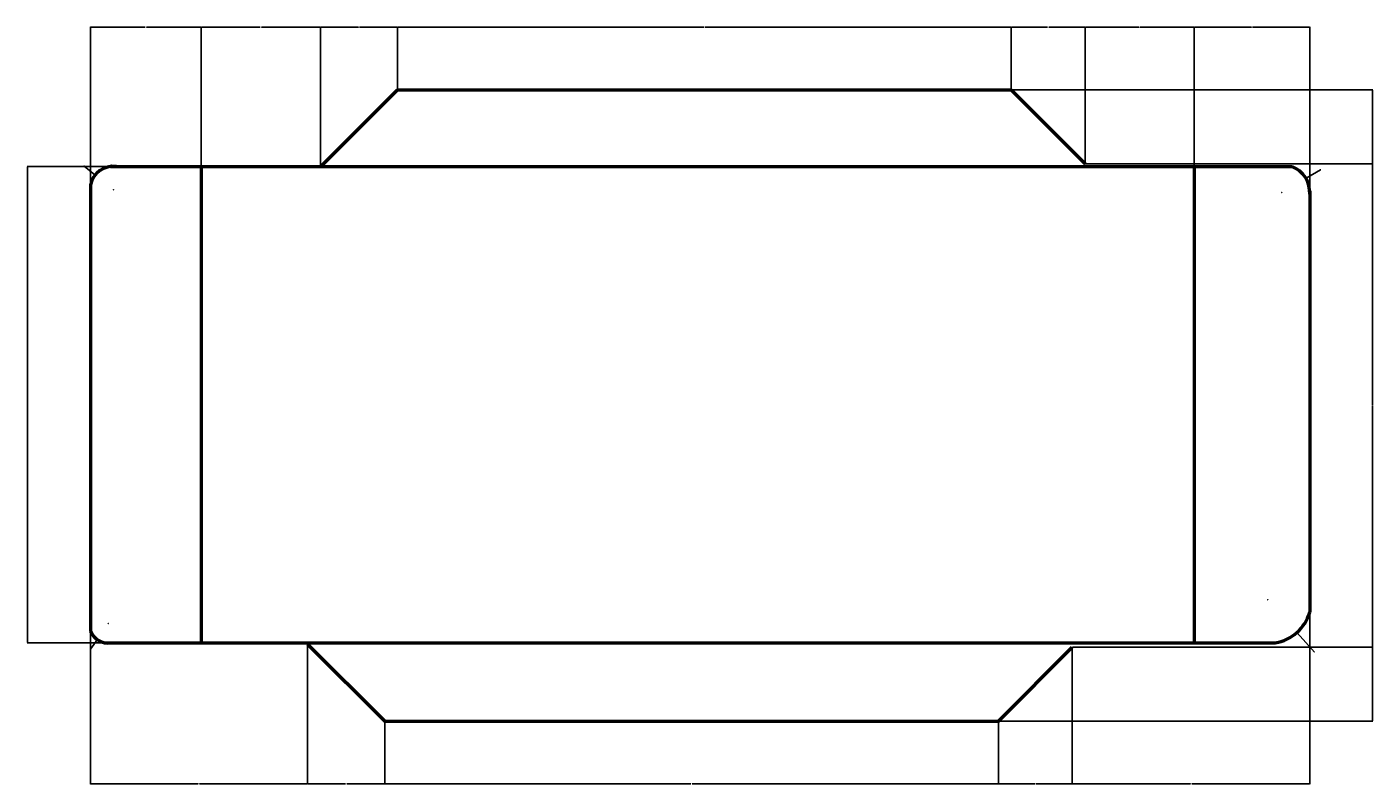
# Model space of a CAD drawing. Units: millimetres. Extents: x 295 to 2981, y 1152 to 2562.
# Tile 1 of 2: x 295 to 1205, y 1853 to 2365. Entities that reach past the tile are written whole.
import ezdxf

# ---------------------------------------------------------------- set-up
doc = ezdxf.new("R2010")
doc.units = ezdxf.units.MM
doc.layers.add('M-DIMS', color=2, linetype='Continuous', lineweight=18)
doc.layers.add('M-OUTL', color=7, linetype='Continuous', lineweight=50)
doc.styles.get("Standard").update_dxf_attribs({"font": 'arial.ttf'})
doc.dimstyles.get("Standard").update_dxf_attribs({"dimtxt": 0.18, "dimasz": 0.18, "dimexe": 0.18, "dimexo": 0.0625, "dimgap": 0.09, "dimtad": 0, "dimtih": 1, "dimtoh": 1, "dimdec": 4, "dimzin": 0, "dimdsep": 46, "dimtxsty": 'Standard', "dimcen": 0.09, "dimadec": 0, "dimazin": 0, "dimtfac": 1, "dimtdec": 4, "dimtofl": 0, "dimtmove": 0, "dimatfit": 3, "dimfxl": 1, "dimtolj": 1, "dimtzin": 0, "dimarcsym": 0})

# ---------------------------------------------------------------- blocks, each defined once
blk = doc.blocks.new('*D10')
at = {"layer": 'Defpoints', "color": 0, "transparency": 16777216}
for p in [(337.98, 1956.62), (484.83, 1947.9), (484.83, 1853.3)]:
    blk.add_point(p, dxfattribs=at)
at = {"layer": 'M-DIMS', "color": 0, "lineweight": -2, "transparency": 16777216}
for p, q in [((337.98, 1956.56), (337.98, 1853.12)), ((484.83, 1947.84), (484.83, 1853.12)), ((338.16, 1853.3), (410.95, 1853.3)), ((484.65, 1853.3), (411.86, 1853.3))]:
    blk.add_line(p, q, dxfattribs=at)
at = {"layer": 'M-DIMS', "color": 0, "transparency": 16777216}
for points in [[(338.16, 1853.33), (338.16, 1853.27), (337.98, 1853.3)], [(484.65, 1853.33), (484.65, 1853.27), (484.83, 1853.3)]]:
    blk.add_solid(points, dxfattribs=at)
at = {"layer": 'M-DIMS', "color": 0, "transparency": 16777216, "insert": (411.41, 1853.3), "char_height": 0.18, "attachment_point": 5}
blk.add_mtext('\\A1;146.84', dxfattribs=at)
blk = doc.blocks.new('*D11')
at = {"layer": 'Defpoints', "color": 0, "transparency": 16777216}
for p in [(484.83, 1947.9), (536.96, 1895.8), (536.96, 1853.3)]:
    blk.add_point(p, dxfattribs=at)
at = {"layer": 'M-DIMS', "color": 0, "lineweight": -2, "transparency": 16777216}
for p, q in [((484.83, 1947.84), (484.83, 1853.12)), ((536.96, 1895.74), (536.96, 1853.12)), ((485.01, 1853.3), (510.5, 1853.3)), ((536.78, 1853.3), (511.29, 1853.3))]:
    blk.add_line(p, q, dxfattribs=at)
at = {"layer": 'M-DIMS', "color": 0, "transparency": 16777216}
for points in [[(485.01, 1853.33), (485.01, 1853.27), (484.83, 1853.3)], [(536.78, 1853.33), (536.78, 1853.27), (536.96, 1853.3)]]:
    blk.add_solid(points, dxfattribs=at)
at = {"layer": 'M-DIMS', "color": 0, "transparency": 16777216, "insert": (510.89, 1853.3), "char_height": 0.18, "attachment_point": 5}
blk.add_mtext('\\A1;52.14', dxfattribs=at)
blk = doc.blocks.new('*D12')
at = {"layer": 'Defpoints', "color": 0, "transparency": 16777216}
for p in [(536.96, 1895.8), (951.87, 1895.8), (951.87, 1853.3)]:
    blk.add_point(p, dxfattribs=at)
at = {"layer": 'M-DIMS', "color": 0, "lineweight": -2, "transparency": 16777216}
for p, q in [((536.96, 1895.74), (536.96, 1853.12)), ((951.87, 1895.74), (951.87, 1853.12)), ((537.14, 1853.3), (744.02, 1853.3)), ((951.69, 1853.3), (744.81, 1853.3))]:
    blk.add_line(p, q, dxfattribs=at)
at = {"layer": 'M-DIMS', "color": 0, "transparency": 16777216}
for points in [[(537.14, 1853.33), (537.14, 1853.27), (536.96, 1853.3)], [(951.69, 1853.33), (951.69, 1853.27), (951.87, 1853.3)]]:
    blk.add_solid(points, dxfattribs=at)
at = {"layer": 'M-DIMS', "color": 0, "transparency": 16777216, "insert": (744.42, 1853.3), "char_height": 0.18, "attachment_point": 5}
blk.add_mtext('\\A1;414.9', dxfattribs=at)
blk = doc.blocks.new('*D13')
at = {"layer": 'Defpoints', "color": 0, "transparency": 16777216}
for p in [(1001.83, 1945.73), (951.87, 1895.8), (1001.83, 1853.3)]:
    blk.add_point(p, dxfattribs=at)
at = {"layer": 'M-DIMS', "color": 0, "lineweight": -2, "transparency": 16777216}
for p, q in [((1001.83, 1945.67), (1001.83, 1853.12)), ((951.87, 1895.74), (951.87, 1853.12)), ((952.05, 1853.3), (976.46, 1853.3)), ((1001.65, 1853.3), (977.25, 1853.3))]:
    blk.add_line(p, q, dxfattribs=at)
at = {"layer": 'M-DIMS', "color": 0, "transparency": 16777216}
for points in [[(952.05, 1853.33), (952.05, 1853.27), (951.87, 1853.3)], [(1001.65, 1853.33), (1001.65, 1853.27), (1001.83, 1853.3)]]:
    blk.add_solid(points, dxfattribs=at)
at = {"layer": 'M-DIMS', "color": 0, "transparency": 16777216, "insert": (976.85, 1853.3), "char_height": 0.18, "attachment_point": 5}
blk.add_mtext('\\A1;49.96', dxfattribs=at)
blk = doc.blocks.new('*D14')
at = {"layer": 'Defpoints', "color": 0, "transparency": 16777216}
for p in [(1162.36, 1969.34), (1001.83, 1945.73), (1162.36, 1853.3)]:
    blk.add_point(p, dxfattribs=at)
at = {"layer": 'M-DIMS', "color": 0, "lineweight": -2, "transparency": 16777216}
for p, q in [((1162.36, 1969.28), (1162.36, 1853.12)), ((1001.83, 1945.67), (1001.83, 1853.12)), ((1002.01, 1853.3), (1081.64, 1853.3)), ((1162.18, 1853.3), (1082.55, 1853.3))]:
    blk.add_line(p, q, dxfattribs=at)
at = {"layer": 'M-DIMS', "color": 0, "transparency": 16777216}
for points in [[(1002.01, 1853.33), (1002.01, 1853.27), (1001.83, 1853.3)], [(1162.18, 1853.33), (1162.18, 1853.27), (1162.36, 1853.3)]]:
    blk.add_solid(points, dxfattribs=at)
at = {"layer": 'M-DIMS', "color": 0, "transparency": 16777216, "insert": (1082.1, 1853.3), "char_height": 0.18, "attachment_point": 5}
blk.add_mtext('\\A1;160.53', dxfattribs=at)
blk = doc.blocks.new('*D15')
at = {"layer": 'Defpoints', "color": 0, "transparency": 16777216}
for p in [(412.93, 2365.26), (412.93, 2271), (337.98, 2258.5)]:
    blk.add_point(p, dxfattribs=at)
at = {"layer": 'M-DIMS', "color": 0, "lineweight": -2, "transparency": 16777216}
for p, q in [((337.98, 2258.56), (337.98, 2365.44)), ((338.16, 2365.26), (375.06, 2365.26)), ((412.75, 2365.26), (375.85, 2365.26)), ((412.93, 2271.06), (412.93, 2365.44))]:
    blk.add_line(p, q, dxfattribs=at)
at = {"layer": 'M-DIMS', "color": 0, "transparency": 16777216}
for points in [[(338.16, 2365.29), (338.16, 2365.23), (337.98, 2365.26)], [(412.75, 2365.29), (412.75, 2365.23), (412.93, 2365.26)]]:
    blk.add_solid(points, dxfattribs=at)
at = {"layer": 'M-DIMS', "color": 0, "transparency": 16777216, "insert": (375.46, 2365.26), "char_height": 0.18, "attachment_point": 5}
blk.add_mtext('\\A1;74.94', dxfattribs=at)
blk = doc.blocks.new('*D16')
at = {"layer": 'Defpoints', "color": 0, "transparency": 16777216}
for p in [(493.52, 2365.26), (412.93, 2271), (493.52, 2270.66)]:
    blk.add_point(p, dxfattribs=at)
at = {"layer": 'M-DIMS', "color": 0, "lineweight": -2, "transparency": 16777216}
for p, q in [((412.93, 2271.06), (412.93, 2365.44)), ((413.11, 2365.26), (452.83, 2365.26)), ((493.34, 2365.26), (453.62, 2365.26)), ((493.52, 2270.72), (493.52, 2365.44))]:
    blk.add_line(p, q, dxfattribs=at)
at = {"layer": 'M-DIMS', "color": 0, "transparency": 16777216}
for points in [[(413.11, 2365.29), (413.11, 2365.23), (412.93, 2365.26)], [(493.34, 2365.29), (493.34, 2365.23), (493.52, 2365.26)]]:
    blk.add_solid(points, dxfattribs=at)
at = {"layer": 'M-DIMS', "color": 0, "transparency": 16777216, "insert": (453.22, 2365.26), "char_height": 0.18, "attachment_point": 5}
blk.add_mtext('\\A1;80.59', dxfattribs=at)
blk = doc.blocks.new('*D17')
at = {"layer": 'Defpoints', "color": 0, "transparency": 16777216}
for p in [(545.65, 2365.26), (545.65, 2322.76), (493.52, 2270.66)]:
    blk.add_point(p, dxfattribs=at)
at = {"layer": 'M-DIMS', "color": 0, "lineweight": -2, "transparency": 16777216}
for p, q in [((493.52, 2270.72), (493.52, 2365.44)), ((493.7, 2365.26), (519.19, 2365.26)), ((545.47, 2365.26), (519.98, 2365.26)), ((545.65, 2322.82), (545.65, 2365.44))]:
    blk.add_line(p, q, dxfattribs=at)
at = {"layer": 'M-DIMS', "color": 0, "transparency": 16777216}
for points in [[(493.7, 2365.29), (493.7, 2365.23), (493.52, 2365.26)], [(545.47, 2365.29), (545.47, 2365.23), (545.65, 2365.26)]]:
    blk.add_solid(points, dxfattribs=at)
at = {"layer": 'M-DIMS', "color": 0, "transparency": 16777216, "insert": (519.58, 2365.26), "char_height": 0.18, "attachment_point": 5}
blk.add_mtext('\\A1;52.14', dxfattribs=at)
blk = doc.blocks.new('*D18')
at = {"layer": 'Defpoints', "color": 0, "transparency": 16777216}
for p in [(960.56, 2365.26), (545.65, 2322.76), (960.56, 2322.76)]:
    blk.add_point(p, dxfattribs=at)
at = {"layer": 'M-DIMS', "color": 0, "lineweight": -2, "transparency": 16777216}
for p, q in [((545.65, 2322.82), (545.65, 2365.44)), ((545.83, 2365.26), (752.71, 2365.26)), ((960.38, 2365.26), (753.5, 2365.26)), ((960.56, 2322.82), (960.56, 2365.44))]:
    blk.add_line(p, q, dxfattribs=at)
at = {"layer": 'M-DIMS', "color": 0, "transparency": 16777216}
for points in [[(545.83, 2365.29), (545.83, 2365.23), (545.65, 2365.26)], [(960.38, 2365.29), (960.38, 2365.23), (960.56, 2365.26)]]:
    blk.add_solid(points, dxfattribs=at)
at = {"layer": 'M-DIMS', "color": 0, "transparency": 16777216, "insert": (753.11, 2365.26), "char_height": 0.18, "attachment_point": 5}
blk.add_mtext('\\A1;414.9', dxfattribs=at)
blk = doc.blocks.new('*D19')
at = {"layer": 'Defpoints', "color": 0, "transparency": 16777216}
for p in [(1010.52, 2365.26), (960.56, 2322.76), (1010.52, 2272.83)]:
    blk.add_point(p, dxfattribs=at)
at = {"layer": 'M-DIMS', "color": 0, "lineweight": -2, "transparency": 16777216}
for p, q in [((960.56, 2322.82), (960.56, 2365.44)), ((960.74, 2365.26), (985.15, 2365.26)), ((1010.34, 2365.26), (985.94, 2365.26)), ((1010.52, 2272.89), (1010.52, 2365.44))]:
    blk.add_line(p, q, dxfattribs=at)
at = {"layer": 'M-DIMS', "color": 0, "transparency": 16777216}
for points in [[(960.74, 2365.29), (960.74, 2365.23), (960.56, 2365.26)], [(1010.34, 2365.29), (1010.34, 2365.23), (1010.52, 2365.26)]]:
    blk.add_solid(points, dxfattribs=at)
at = {"layer": 'M-DIMS', "color": 0, "transparency": 16777216, "insert": (985.54, 2365.26), "char_height": 0.18, "attachment_point": 5}
blk.add_mtext('\\A1;49.96', dxfattribs=at)
blk = doc.blocks.new('*D20')
at = {"layer": 'Defpoints', "color": 0, "transparency": 16777216}
for p in [(1084.16, 2365.26), (1010.52, 2272.83), (1084.16, 2271)]:
    blk.add_point(p, dxfattribs=at)
at = {"layer": 'M-DIMS', "color": 0, "lineweight": -2, "transparency": 16777216}
for p, q in [((1010.52, 2272.89), (1010.52, 2365.44)), ((1010.7, 2365.26), (1046.95, 2365.26)), ((1083.98, 2365.26), (1047.73, 2365.26)), ((1084.16, 2271.06), (1084.16, 2365.44))]:
    blk.add_line(p, q, dxfattribs=at)
at = {"layer": 'M-DIMS', "color": 0, "transparency": 16777216}
for points in [[(1010.7, 2365.29), (1010.7, 2365.23), (1010.52, 2365.26)], [(1083.98, 2365.29), (1083.98, 2365.23), (1084.16, 2365.26)]]:
    blk.add_solid(points, dxfattribs=at)
at = {"layer": 'M-DIMS', "color": 0, "transparency": 16777216, "insert": (1047.34, 2365.26), "char_height": 0.18, "attachment_point": 5}
blk.add_mtext('\\A1;73.64', dxfattribs=at)
blk = doc.blocks.new('*D21')
at = {"layer": 'Defpoints', "color": 0, "transparency": 16777216}
for p in [(1162.36, 2365.26), (1084.16, 2271), (1162.36, 2252.23)]:
    blk.add_point(p, dxfattribs=at)
at = {"layer": 'M-DIMS', "color": 0, "lineweight": -2, "transparency": 16777216}
for p, q in [((1084.16, 2271.06), (1084.16, 2365.44)), ((1084.34, 2365.26), (1122.94, 2365.26)), ((1162.18, 2365.26), (1123.58, 2365.26)), ((1162.36, 2252.29), (1162.36, 2365.44))]:
    blk.add_line(p, q, dxfattribs=at)
at = {"layer": 'M-DIMS', "color": 0, "transparency": 16777216}
for points in [[(1084.34, 2365.29), (1084.34, 2365.23), (1084.16, 2365.26)], [(1162.18, 2365.29), (1162.18, 2365.23), (1162.36, 2365.26)]]:
    blk.add_solid(points, dxfattribs=at)
at = {"layer": 'M-DIMS', "color": 0, "transparency": 16777216, "insert": (1123.26, 2365.26), "char_height": 0.18, "attachment_point": 5}
blk.add_mtext('\\A1;78.2', dxfattribs=at)
blk = doc.blocks.new('*D22')
at = {"layer": 'Defpoints', "color": 0, "transparency": 16777216}
for p in [(960.56, 2322.76), (951.87, 1895.8), (1204.86, 1895.8)]:
    blk.add_point(p, dxfattribs=at)
at = {"layer": 'M-DIMS', "color": 0, "lineweight": -2, "transparency": 16777216}
for p, q in [((960.62, 2322.76), (1205.04, 2322.76)), ((1204.86, 2322.58), (1204.86, 2109.46)), ((1204.86, 1895.98), (1204.86, 2109.1)), ((951.93, 1895.8), (1205.04, 1895.8))]:
    blk.add_line(p, q, dxfattribs=at)
at = {"layer": 'M-DIMS', "color": 0, "transparency": 16777216}
for points in [[(1204.83, 2322.58), (1204.89, 2322.58), (1204.86, 2322.76)], [(1204.83, 1895.98), (1204.89, 1895.98), (1204.86, 1895.8)]]:
    blk.add_solid(points, dxfattribs=at)
at = {"layer": 'M-DIMS', "color": 0, "transparency": 16777216, "insert": (1204.86, 2109.28), "char_height": 0.18, "attachment_point": 5}
blk.add_mtext('\\A1;427', dxfattribs=at)
blk = doc.blocks.new('*D23')
at = {"layer": 'Defpoints', "color": 0, "transparency": 16777216}
for p in [(960.56, 2322.76), (1204.86, 2322.76), (1010.52, 2272.83)]:
    blk.add_point(p, dxfattribs=at)
at = {"layer": 'M-DIMS', "color": 0, "lineweight": -2, "transparency": 16777216}
for p, q in [((960.62, 2322.76), (1205.04, 2322.76)), ((1204.86, 2322.58), (1204.86, 2297.98)), ((1204.86, 2273.01), (1204.86, 2297.61)), ((1010.59, 2272.83), (1205.04, 2272.83))]:
    blk.add_line(p, q, dxfattribs=at)
at = {"layer": 'M-DIMS', "color": 0, "transparency": 16777216}
for points in [[(1204.83, 2322.58), (1204.89, 2322.58), (1204.86, 2322.76)], [(1204.83, 2273.01), (1204.89, 2273.01), (1204.86, 2272.83)]]:
    blk.add_solid(points, dxfattribs=at)
at = {"layer": 'M-DIMS', "color": 0, "transparency": 16777216, "insert": (1204.86, 2297.79), "char_height": 0.18, "attachment_point": 5}
blk.add_mtext('\\A1;49.93', dxfattribs=at)
blk = doc.blocks.new('*D24')
at = {"layer": 'Defpoints', "color": 0, "transparency": 16777216}
for p in [(1001.83, 1945.73), (951.87, 1895.8), (1204.86, 1895.8)]:
    blk.add_point(p, dxfattribs=at)
at = {"layer": 'M-DIMS', "color": 0, "lineweight": -2, "transparency": 16777216}
for p, q in [((1001.9, 1945.73), (1205.04, 1945.73)), ((1204.86, 1945.55), (1204.86, 1920.95)), ((1204.86, 1895.98), (1204.86, 1920.58)), ((951.93, 1895.8), (1205.04, 1895.8))]:
    blk.add_line(p, q, dxfattribs=at)
at = {"layer": 'M-DIMS', "color": 0, "transparency": 16777216}
for points in [[(1204.83, 1945.55), (1204.89, 1945.55), (1204.86, 1945.73)], [(1204.83, 1895.98), (1204.89, 1895.98), (1204.86, 1895.8)]]:
    blk.add_solid(points, dxfattribs=at)
at = {"layer": 'M-DIMS', "color": 0, "transparency": 16777216, "insert": (1204.86, 1920.76), "char_height": 0.18, "attachment_point": 5}
blk.add_mtext('\\A1;49.93', dxfattribs=at)
blk = doc.blocks.new('*D25')
at = {"layer": 'Defpoints', "color": 0, "transparency": 16777216}
for p in [(295.48, 2271), (412.93, 2271), (412.93, 1948.64)]:
    blk.add_point(p, dxfattribs=at)
at = {"layer": 'M-DIMS', "color": 0, "lineweight": -2, "transparency": 16777216}
for p, q in [((412.87, 2271), (295.3, 2271)), ((295.48, 2270.82), (295.48, 2110)), ((295.48, 1948.82), (295.48, 2109.64)), ((412.87, 1948.64), (295.3, 1948.64))]:
    blk.add_line(p, q, dxfattribs=at)
at = {"layer": 'M-DIMS', "color": 0, "transparency": 16777216}
for points in [[(295.45, 2270.82), (295.51, 2270.82), (295.48, 2271)], [(295.45, 1948.82), (295.51, 1948.82), (295.48, 1948.64)]]:
    blk.add_solid(points, dxfattribs=at)
at = {"layer": 'M-DIMS', "color": 0, "transparency": 16777216, "insert": (295.48, 2109.82), "char_height": 0.18, "attachment_point": 5}
blk.add_mtext('\\A1;322.35', dxfattribs=at)
blk = doc.blocks.new('*D48')
at = {"layer": 'Defpoints', "color": 0, "transparency": 16777216}
for p in [(1133.97, 1977.83), (1153.66, 1955.69)]:
    blk.add_point(p, dxfattribs=at)
at = {"layer": 'M-DIMS', "color": 0, "lineweight": -2, "transparency": 16777216}
for p, q in [((1133.88, 1977.83), (1134.06, 1977.83)), ((1133.97, 1977.74), (1133.97, 1977.92)), ((1165.48, 1942.4), (1153.78, 1955.55)), ((1165.66, 1942.4), (1165.48, 1942.4))]:
    blk.add_line(p, q, dxfattribs=at)
at = {"layer": 'M-DIMS', "color": 0, "transparency": 16777216}
blk.add_solid([(1153.8, 1955.57), (1153.76, 1955.53), (1153.66, 1955.69)], dxfattribs=at)
at = {"layer": 'M-DIMS', "color": 0, "transparency": 16777216, "insert": (1166.21, 1942.4), "char_height": 0.18, "attachment_point": 5}
blk.add_mtext('\\A1;R29.636', dxfattribs=at)
blk = doc.blocks.new('*D49')
at = {"layer": 'Defpoints', "color": 0, "transparency": 16777216}
for p in [(341.21, 2265.27), (353.54, 2255.23)]:
    blk.add_point(p, dxfattribs=at)
at = {"layer": 'M-DIMS', "color": 0, "lineweight": -2, "transparency": 16777216}
for p, q in [((333.64, 2271.29), (333.82, 2271.29)), ((333.82, 2271.29), (341.07, 2265.38)), ((353.45, 2255.23), (353.63, 2255.23)), ((353.54, 2255.14), (353.54, 2255.32))]:
    blk.add_line(p, q, dxfattribs=at)
at = {"layer": 'M-DIMS', "color": 0, "transparency": 16777216}
blk.add_solid([(341.09, 2265.4), (341.06, 2265.36), (341.21, 2265.27)], dxfattribs=at)
at = {"layer": 'M-DIMS', "color": 0, "transparency": 16777216, "insert": (333.09, 2271.29), "char_height": 0.18, "attachment_point": 5}
blk.add_mtext('\\A1;R15.897', dxfattribs=at)
blk = doc.blocks.new('*D50')
at = {"layer": 'Defpoints', "color": 0, "transparency": 16777216}
for p in [(1159.81, 2262.89), (1143.42, 2253.33)]:
    blk.add_point(p, dxfattribs=at)
at = {"layer": 'M-DIMS', "color": 0, "lineweight": -2, "transparency": 16777216}
for p, q in [((1169.64, 2268.62), (1159.96, 2262.98)), ((1169.82, 2268.62), (1169.64, 2268.62)), ((1143.33, 2253.33), (1143.51, 2253.33)), ((1143.42, 2253.24), (1143.42, 2253.42))]:
    blk.add_line(p, q, dxfattribs=at)
at = {"layer": 'M-DIMS', "color": 0, "transparency": 16777216}
blk.add_solid([(1159.95, 2263), (1159.98, 2262.95), (1159.81, 2262.89)], dxfattribs=at)
at = {"layer": 'M-DIMS', "color": 0, "transparency": 16777216, "insert": (1170.3, 2268.62), "char_height": 0.18, "attachment_point": 5}
blk.add_mtext('\\A1;R18.97', dxfattribs=at)
blk = doc.blocks.new('*D51')
at = {"layer": 'Defpoints', "color": 0, "transparency": 16777216}
for p in [(350.14, 1961.68), (342.61, 1950.88)]:
    blk.add_point(p, dxfattribs=at)
at = {"layer": 'M-DIMS', "color": 0, "lineweight": -2, "transparency": 16777216}
for p, q in [((350.05, 1961.68), (350.23, 1961.68)), ((350.14, 1961.59), (350.14, 1961.77)), ((338.09, 1944.39), (342.51, 1950.73)), ((337.91, 1944.39), (338.09, 1944.39))]:
    blk.add_line(p, q, dxfattribs=at)
at = {"layer": 'M-DIMS', "color": 0, "transparency": 16777216}
blk.add_solid([(342.48, 1950.75), (342.53, 1950.71), (342.61, 1950.88)], dxfattribs=at)
at = {"layer": 'M-DIMS', "color": 0, "transparency": 16777216, "insert": (337.36, 1944.39), "char_height": 0.18, "attachment_point": 5}
blk.add_mtext('\\A1;R13.172', dxfattribs=at)

msp = doc.modelspace()

# ---------------------------------------------------------------- linework, layer by layer
at = {"layer": 'M-OUTL'}
for p, q in [((493.5164, 2270.6595), (545.6516, 2322.758)), ((545.6516, 2322.758), (912.7704, 2322.758)), ((912.7704, 2322.758), (960.561, 2322.758)), ((960.561, 2322.758), (1010.5239, 2272.8303)), ((351.503, 2270.997), (1150.321, 2270.997)), ((412.9282, 2270.997), (412.9282, 1948.642)), ((1084.159, 2270.997), (1084.159, 1948.642)), ((337.9849, 2258.4984), (337.9849, 1956.6175)), ((1162.3606, 2254.4235), (1162.3606, 1969.3422)), ((348.2832, 1948.642), (1139.0856, 1948.642)), ((484.8272, 1947.8989), (536.9624, 1895.8003)), ((951.8717, 1895.8003), (1001.8347, 1945.7281)), ((536.9624, 1895.8003), (904.0812, 1895.8003)), ((904.0812, 1895.8003), (951.8717, 1895.8003))]:
    msp.add_line(p, q, dxfattribs=at)
for centre, radius, start, end in [((353.5426, 2255.2314), 15.897, 82.628502, 168.1403973), ((1143.4224, 2253.3258), 18.97, 356.6827563, 68.6748388), ((1133.9672, 1977.8322), 29.6356, 279.9454661, 343.3526661), ((350.1443, 1961.6816), 13.1717, 202.610509, 278.1228545)]:
    msp.add_arc(centre, radius, start, end, dxfattribs=at)

# ---------------------------------------------------------------- dimensions: what is measured, and where the dimension line sits
at = {"layer": 'M-DIMS'}
for base, p1, p2, override, picture, middle in [((412.9282, 2365.258), (337.9849, 2258.4984), (412.9282, 2270.997), {"dimdec": 2, "dimlfac": 1, "dimrnd": 0, "dimzin": 0, "dimdsep": 46, "dimlunit": 2}, '*D15', (375.4566, 2365.258)), ((493.5164, 2365.258), (412.9282, 2270.997), (493.5164, 2270.6595), {"dimdec": 2, "dimlfac": 1, "dimrnd": 0, "dimzin": 0, "dimdsep": 46, "dimlunit": 2}, '*D16', (453.2223, 2365.258)), ((545.6516, 2365.258), (493.5164, 2270.6595), (545.6516, 2322.758), {"dimdec": 2, "dimlfac": 1, "dimrnd": 0, "dimzin": 0, "dimdsep": 46, "dimlunit": 2}, '*D17', (519.584, 2365.258)), ((960.561, 2365.258), (545.6516, 2322.758), (960.561, 2322.758), {"dimdec": 1, "dimlfac": 1, "dimrnd": 0, "dimzin": 0, "dimdsep": 46, "dimlunit": 2}, '*D18', (753.1063, 2365.258)), ((1010.5239, 2365.258), (960.561, 2322.758), (1010.5239, 2272.8303), {"dimdec": 2, "dimlfac": 1, "dimrnd": 0, "dimzin": 0, "dimdsep": 46, "dimlunit": 2}, '*D19', (985.5424, 2365.258)), ((1084.159, 2365.258), (1010.5239, 2272.8303), (1084.159, 2270.997), {"dimdec": 2, "dimlfac": 1, "dimrnd": 0, "dimzin": 0, "dimdsep": 46, "dimlunit": 2}, '*D20', (1047.3414, 2365.258)), ((1162.3606, 2365.258), (1084.159, 2270.997), (1162.3606, 2252.2281), {"dimdec": 1, "dimlfac": 1, "dimrnd": 0, "dimzin": 0, "dimdsep": 46, "dimlunit": 2}, '*D21', (1123.2598, 2365.258)), ((1162.3606, 1853.3003), (1001.8347, 1945.7281), (1162.3606, 1969.3422), {"dimdec": 2, "dimlfac": 1, "dimrnd": 0, "dimzin": 0, "dimdsep": 46, "dimlunit": 2}, '*D14', (1082.0976, 1853.3003)), ((484.8272, 1853.3003), (337.9849, 1956.6175), (484.8272, 1947.8989), {"dimdec": 2, "dimlfac": 1, "dimrnd": 0, "dimzin": 0, "dimdsep": 46, "dimlunit": 2}, '*D10', (411.4061, 1853.3003)), ((536.9624, 1853.3003), (484.8272, 1947.8989), (536.9624, 1895.8003), {"dimdec": 2, "dimlfac": 1, "dimrnd": 0, "dimzin": 0, "dimdsep": 46, "dimlunit": 2}, '*D11', (510.8948, 1853.3003)), ((1001.8347, 1853.3003), (951.8717, 1895.8003), (1001.8347, 1945.7281), {"dimdec": 2, "dimlfac": 1, "dimrnd": 0, "dimzin": 0, "dimdsep": 46, "dimlunit": 2}, '*D13', (976.8532, 1853.3003)), ((951.8717, 1853.3003), (536.9624, 1895.8003), (951.8717, 1895.8003), {"dimdec": 1, "dimlfac": 1, "dimrnd": 0, "dimzin": 0, "dimdsep": 46, "dimlunit": 2}, '*D12', (744.4171, 1853.3003))]:
    dim = msp.add_linear_dim(base=base, p1=p1, p2=p2, dimstyle='Standard', override=override, dxfattribs=at)
    dim.commit()
    dim.dimension.update_dxf_attribs({"geometry": picture, "text_midpoint": middle})
for base, p1, p2, override, picture, middle in [((1204.8606, 1895.8003), (960.561, 2322.758), (951.8717, 1895.8003), {"dimdec": 0, "dimlfac": 1, "dimrnd": 0, "dimzin": 0, "dimdsep": 46, "dimlunit": 2}, '*D22', (1204.8606, 2109.2792)), ((1204.8606, 2322.758), (1010.5239, 2272.8303), (960.561, 2322.758), {"dimdec": 2, "dimlfac": 1, "dimrnd": 0, "dimzin": 0, "dimdsep": 46, "dimlunit": 2}, '*D23', (1204.8606, 2297.7941)), ((295.48493, 2270.99696), (412.92818, 1948.64202), (412.92818, 2270.99696), {"dimdec": 2, "dimlfac": 1, "dimrnd": 0, "dimzin": 0, "dimdsep": 46, "dimlunit": 2}, '*D25', (295.48493, 2109.81949)), ((1204.8606, 1895.8003), (1001.8347, 1945.7281), (951.8717, 1895.8003), {"dimdec": 2, "dimlfac": 1, "dimrnd": 0, "dimzin": 0, "dimdsep": 46, "dimlunit": 2}, '*D24', (1204.8606, 1920.7642))]:
    dim = msp.add_linear_dim(base=base, p1=p1, p2=p2, angle=90, dimstyle='Standard', override=override, dxfattribs=at)
    dim.commit()
    dim.dimension.update_dxf_attribs({"geometry": picture, "text_midpoint": middle})
for center, mpoint, override, picture, middle in [((353.5426, 2255.2314), (341.2144, 2265.2678), {"dimdec": 3, "dimlfac": 1, "dimrnd": 0, "dimzin": 0, "dimdsep": 46, "dimlunit": 2}, '*D49', (333.0877, 2271.2896)), ((1143.4224, 2253.3258), (1159.8066, 2262.8871), {"dimdec": 2, "dimlfac": 1, "dimrnd": 0, "dimzin": 0, "dimdsep": 46, "dimlunit": 2}, '*D50', (1170.297, 2268.624)), ((1133.9672, 1977.8322), (1153.6622, 1955.6878), {"dimdec": 3, "dimlfac": 1, "dimrnd": 0, "dimzin": 0, "dimdsep": 46, "dimlunit": 2}, '*D48', (1166.2088, 1942.4012)), ((350.1443, 1961.6816), (342.6112, 1950.8767), {"dimdec": 3, "dimlfac": 1, "dimrnd": 0, "dimzin": 0, "dimdsep": 46, "dimlunit": 2}, '*D51', (337.3625, 1944.3937))]:
    dim = msp.add_radius_dim(center=center, mpoint=mpoint, dimstyle='Standard', override=override, dxfattribs=at)
    dim.commit()
    dim.dimension.update_dxf_attribs({"geometry": picture, "text_midpoint": middle, "dimtype": 164})

doc.saveas('drawing.dxf')
